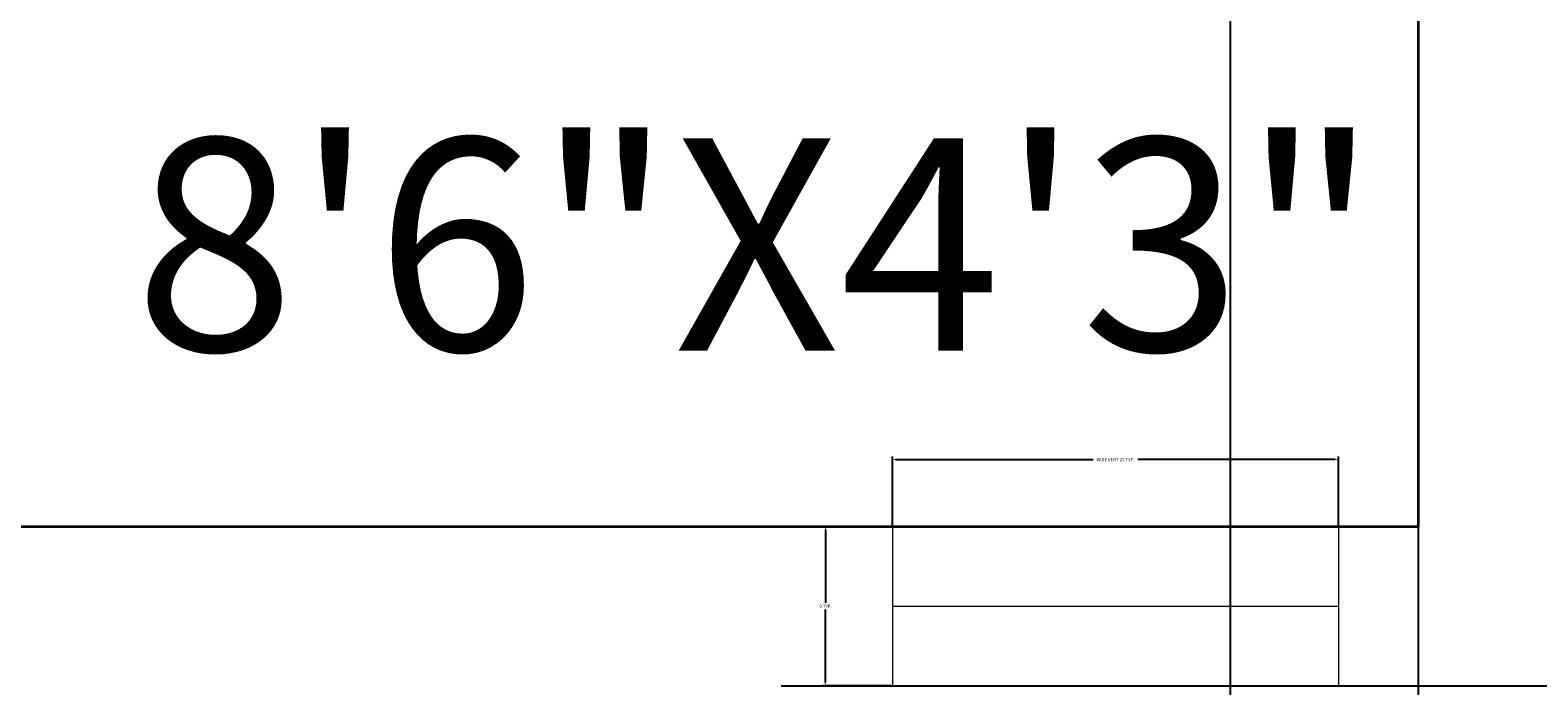
# Model space of a CAD drawing. Units: feet. Extents: x 5816 to 6644, y 25475 to 26788.
# Tile 20 of 23: x 6147 to 6232, y 26499 to 26536. Entities that reach past the tile are written whole.
import ezdxf

# ---------------------------------------------------------------- set-up
doc = ezdxf.new("R2010")
doc.units = ezdxf.units.FT
for name, color, linetype, lineweight in [('A-ANNO-DIMS', 2, 'Continuous', 13), ('A-FLOR-SHFT', 8, 'Continuous', 25), ('A-GLAZ', 4, 'Continuous', 18), ('A-WALL', 7, 'Continuous', 35)]:
    doc.layers.add(name, color=color, linetype=linetype, lineweight=lineweight)
doc.styles.get("Standard").update_dxf_attribs({"font": 'arial.ttf'})
doc.dimstyles.get("Standard").update_dxf_attribs({"dimtxt": 0.18, "dimasz": 0.18, "dimexe": 0.18, "dimexo": 0.0625, "dimgap": 0.09, "dimtad": 0, "dimtih": 1, "dimtoh": 1, "dimdec": 4, "dimzin": 0, "dimdsep": 46, "dimtxsty": 'Standard', "dimcen": 0.09, "dimadec": 0, "dimazin": 0, "dimtfac": 1, "dimtdec": 4, "dimtofl": 0, "dimtmove": 0, "dimatfit": 3, "dimfxl": 1, "dimtolj": 1, "dimtzin": 0, "dimarcsym": 0})

# ---------------------------------------------------------------- blocks, each defined once
blk = doc.blocks.new('WIN-VENT-WIDE')
for p, q in [((0, 0), (0, -9)), ((25.199, 0), (25.199, -9)), ((0, -4.5), (25.199, -4.5))]:
    blk.add_line(p, q)
blk = doc.blocks.new('VENT-SHAFT')
blk.add_line((0, 103), (81, 103))
blk = doc.blocks.new('*D49')
at = {"layer": 'A-ANNO-DIMS', "color": 0, "lineweight": -2, "transparency": 16777216}
for p, q in [((6195.595, 26507.647), (6195.595, 26511.545)), ((6220.794, 26507.647), (6220.794, 26511.545)), ((6195.775, 26511.365), (6206.929, 26511.365)), ((6220.614, 26511.365), (6209.46, 26511.365))]:
    blk.add_line(p, q, dxfattribs=at)
at = {"layer": 'A-ANNO-DIMS', "color": 0, "transparency": 16777216}
for points in [[(6195.775, 26511.395), (6195.775, 26511.335), (6195.595, 26511.365)], [(6220.614, 26511.395), (6220.614, 26511.335), (6220.794, 26511.365)]]:
    blk.add_solid(points, dxfattribs=at)
at = {"layer": 'Defpoints', "color": 0, "transparency": 16777216}
for p in [(6220.794, 26511.365), (6195.595, 26507.585), (6220.794, 26507.585)]:
    blk.add_point(p, dxfattribs=at)
at = {"layer": 'A-ANNO-DIMS', "color": 0, "transparency": 16777216, "insert": (6208.195, 26511.365), "char_height": 0.18, "attachment_point": 5}
blk.add_mtext('\\A1;WIDE VENT 25 TYP.', dxfattribs=at)
blk = doc.blocks.new('*D50')
at = {"layer": 'A-ANNO-DIMS', "color": 0, "lineweight": -2, "transparency": 16777216}
for p, q in [((6195.533, 26507.585), (6191.635, 26507.585)), ((6191.815, 26507.405), (6191.815, 26503.267)), ((6191.815, 26498.765), (6191.815, 26502.903)), ((6195.533, 26498.585), (6191.635, 26498.585))]:
    blk.add_line(p, q, dxfattribs=at)
at = {"layer": 'A-ANNO-DIMS', "color": 0, "transparency": 16777216}
for points in [[(6191.785, 26507.405), (6191.845, 26507.405), (6191.815, 26507.585)], [(6191.785, 26498.765), (6191.845, 26498.765), (6191.815, 26498.585)]]:
    blk.add_solid(points, dxfattribs=at)
at = {"layer": 'Defpoints', "color": 0, "transparency": 16777216}
for p in [(6191.815, 26507.585), (6195.595, 26507.585), (6195.595, 26498.585)]:
    blk.add_point(p, dxfattribs=at)
at = {"layer": 'A-ANNO-DIMS', "color": 0, "transparency": 16777216, "insert": (6191.815, 26503.085), "char_height": 0.18, "attachment_point": 5}
blk.add_mtext('\\A1;9 TYP.', dxfattribs=at)
blk = doc.blocks.new('*D60')
at = {"layer": 'A-ANNO-DIMS', "color": 0, "lineweight": -2, "transparency": 16777216}
for p, q in [((6106.978, 26094.399), (6106.978, 26787.915)), ((6107.158, 26787.735), (6224.932, 26787.735)), ((6343.496, 26787.735), (6225.722, 26787.735)), ((6343.676, 26094.399), (6343.676, 26787.915))]:
    blk.add_line(p, q, dxfattribs=at)
at = {"layer": 'A-ANNO-DIMS', "color": 0, "transparency": 16777216}
for points in [[(6107.158, 26787.765), (6107.158, 26787.705), (6106.978, 26787.735)], [(6343.496, 26787.765), (6343.496, 26787.705), (6343.676, 26787.735)]]:
    blk.add_solid(points, dxfattribs=at)
at = {"layer": 'Defpoints', "color": 0, "transparency": 16777216}
for p in [(6343.676, 26787.735), (6106.978, 26094.337), (6343.676, 26094.337)]:
    blk.add_point(p, dxfattribs=at)
at = {"layer": 'A-ANNO-DIMS', "color": 0, "transparency": 16777216, "insert": (6225.327, 26787.735), "char_height": 0.18, "attachment_point": 5}
blk.add_mtext('\\A1;236.7', dxfattribs=at)
blk = doc.blocks.new('*D72')
at = {"layer": 'A-ANNO-DIMS', "color": 0, "lineweight": -2, "transparency": 16777216}
for p, q in [((6214.691, 26168.647), (6214.691, 26787.915)), ((6214.871, 26787.735), (6219.563, 26787.735)), ((6225.132, 26787.735), (6220.439, 26787.735)), ((6225.312, 26177.647), (6225.312, 26787.915))]:
    blk.add_line(p, q, dxfattribs=at)
at = {"layer": 'A-ANNO-DIMS', "color": 0, "transparency": 16777216}
for points in [[(6214.871, 26787.765), (6214.871, 26787.705), (6214.691, 26787.735)], [(6225.132, 26787.765), (6225.132, 26787.705), (6225.312, 26787.735)]]:
    blk.add_solid(points, dxfattribs=at)
at = {"layer": 'Defpoints', "color": 0, "transparency": 16777216}
for p in [(6225.312, 26787.735), (6225.312, 26177.585), (6214.691, 26168.585)]:
    blk.add_point(p, dxfattribs=at)
at = {"layer": 'A-ANNO-DIMS', "color": 0, "transparency": 16777216, "insert": (6220.001, 26787.735), "char_height": 0.18, "attachment_point": 5}
blk.add_mtext('\\A1;10.621', dxfattribs=at)

msp = doc.modelspace()

# ---------------------------------------------------------------- linework, layer by layer
at = {"layer": 'A-WALL'}
for p, q in [((6225.3119, 26507.5846), (6225.3119, 26558.5846)), ((6123.3119, 26507.5846), (6225.3119, 26507.5846))]:
    msp.add_line(p, q, dxfattribs=at)

# ---------------------------------------------------------------- block references
at = {"layer": 'A-FLOR-SHFT'}
msp.add_blockref('VENT-SHAFT', (6189.3119, 26395.5846), dxfattribs=at)
at = {"layer": 'A-GLAZ'}
msp.add_blockref('WIN-VENT-WIDE', (6195.5951, 26507.5846), dxfattribs=at)

# ---------------------------------------------------------------- texts
at = {"layer": 'A-ANNO-DIMS'}
msp.add_text('8\'6"X4\'3"', height=12, dxfattribs=at).set_placement((6152.7543, 26517.516))

# ---------------------------------------------------------------- dimensions: what is measured, and where the dimension line sits
for base, p1, p2, override, picture, middle in [((6343.6763, 26787.7346), (6106.9781, 26094.3368), (6343.6763, 26094.3368), {"dimdec": 1, "dimlfac": 1, "dimrnd": 0, "dimzin": 0, "dimdsep": 46, "dimlunit": 2}, '*D60', (6225.3272, 26787.7346)), ((6225.3119, 26787.7346), (6214.6905, 26168.5846), (6225.3119, 26177.5846), {"dimdec": 3, "dimlfac": 1, "dimrnd": 0, "dimzin": 0, "dimdsep": 46, "dimlunit": 2}, '*D72', (6220.0012, 26787.7346))]:
    dim = msp.add_linear_dim(base=base, p1=p1, p2=p2, dimstyle='Standard', override=override, dxfattribs=at)
    dim.commit()
    dim.dimension.update_dxf_attribs({"geometry": picture, "text_midpoint": middle})
dim = msp.add_linear_dim(base=(6220.7941, 26511.3645), p1=(6195.5951, 26507.5846), p2=(6220.7941, 26507.5846), text='WIDE VENT <> TYP.', dimstyle='Standard', override={"dimdec": 0, "dimlfac": 1, "dimrnd": 0, "dimzin": 0, "dimdsep": 46, "dimlunit": 2}, dxfattribs=at)
dim.commit()
dim.dimension.update_dxf_attribs({"geometry": '*D49', "text_midpoint": (6208.1946, 26511.3645)})
dim = msp.add_linear_dim(base=(6191.8152, 26507.5846), p1=(6195.5951, 26498.5846), p2=(6195.5951, 26507.5846), angle=90, text='<> TYP.', dimstyle='Standard', override={"dimdec": 0, "dimlfac": 1, "dimrnd": 0, "dimzin": 0, "dimdsep": 46, "dimlunit": 2}, dxfattribs=at)
dim.commit()
dim.dimension.update_dxf_attribs({"geometry": '*D50', "text_midpoint": (6191.8152, 26503.0846)})

doc.saveas('drawing.dxf')
